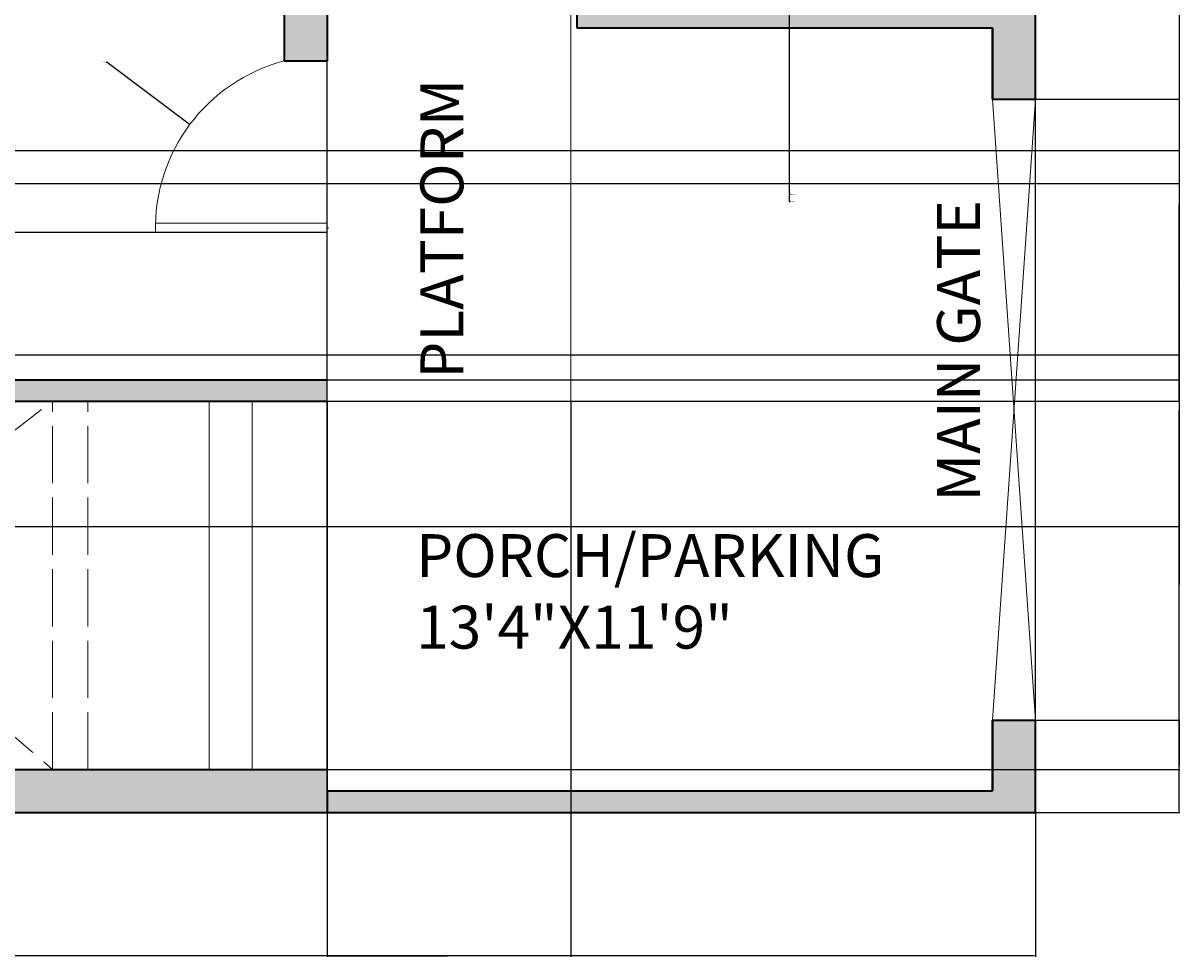
# Model space of a CAD drawing. Units: feet. Extents: x 1699 to 2359, y 1819 to 2211.
# Tile 3 of 4: x 2117 to 2359, y 1819 to 2014. Entities that reach past the tile are written whole.
import ezdxf

# ---------------------------------------------------------------- set-up
doc = ezdxf.new("R2010")
doc.units = ezdxf.units.FT
doc.linetypes.add('ACAD_ISO02W100', pattern=[15, 12, -3])
for name, color, linetype, lineweight in [('A-ANNO-DIMS', 2, 'Continuous', 18), ('A-ANNO-TEXT', 7, 'Continuous', 18), ('A-AREA-IDEN', 7, 'Continuous', 18), ('A-DOOR', 4, 'Continuous', 18), ('A-FLOR', 7, 'Continuous', 18), ('A-FLOR-STRS', 7, 'Continuous', 18), ('A-FLOR-STRS-OVHD', 8, 'ACAD_ISO02W100', 13), ('A-WALL', 7, 'Continuous', 35), ('A-WALL-PATT', 1, 'Continuous', 13)]:
    doc.layers.add(name, color=color, linetype=linetype, lineweight=lineweight)
doc.styles.get("Standard").update_dxf_attribs({"font": 'arial.ttf'})
doc.dimstyles.get("Standard").update_dxf_attribs({"dimtxt": 0.18, "dimasz": 0.18, "dimexe": 0.18, "dimexo": 0.0625, "dimgap": 0.09, "dimtad": 0, "dimtih": 1, "dimtoh": 1, "dimdec": 4, "dimzin": 0, "dimdsep": 46, "dimtxsty": 'Standard', "dimcen": 0.09, "dimadec": 0, "dimazin": 0, "dimtfac": 1, "dimtdec": 4, "dimtofl": 0, "dimtmove": 0, "dimatfit": 3, "dimfxl": 1, "dimtolj": 1, "dimtzin": 0, "dimarcsym": 0})

# ---------------------------------------------------------------- blocks, each defined once
blk = doc.blocks.new('*D22')
at = {"layer": 'A-ANNO-DIMS', "color": 0, "lineweight": -2, "transparency": 16777216}
for p, q in [((2180.43, 1853.41), (2180.43, 2210.63)), ((2180.61, 2210.45), (2254.29, 2210.45)), ((2328.75, 2210.45), (2255.06, 2210.45)), ((2328.93, 1848.91), (2328.93, 2210.63))]:
    blk.add_line(p, q, dxfattribs=at)
at = {"layer": 'A-ANNO-DIMS', "color": 0, "transparency": 16777216}
for points in [[(2180.61, 2210.48), (2180.61, 2210.42), (2180.43, 2210.45)], [(2328.75, 2210.48), (2328.75, 2210.42), (2328.93, 2210.45)]]:
    blk.add_solid(points, dxfattribs=at)
at = {"layer": 'Defpoints', "color": 0, "transparency": 16777216}
for p in [(2328.93, 2210.45), (2180.43, 1853.35), (2328.93, 1848.85)]:
    blk.add_point(p, dxfattribs=at)
at = {"layer": 'A-ANNO-DIMS', "color": 0, "transparency": 16777216, "insert": (2254.68, 2210.45), "char_height": 0.18, "attachment_point": 5}
blk.add_mtext('\\A1;148.5', dxfattribs=at)
blk = doc.blocks.new('*D23')
at = {"layer": 'A-ANNO-DIMS', "color": 0, "lineweight": -2, "transparency": 16777216}
for p, q in [((1955.43, 1857.79), (1955.43, 1818.57)), ((2180.43, 1857.79), (2180.43, 1818.57)), ((1955.61, 1818.75), (2067.64, 1818.75)), ((2180.25, 1818.75), (2068.22, 1818.75))]:
    blk.add_line(p, q, dxfattribs=at)
at = {"layer": 'A-ANNO-DIMS', "color": 0, "transparency": 16777216}
for points in [[(1955.61, 1818.78), (1955.61, 1818.72), (1955.43, 1818.75)], [(2180.25, 1818.78), (2180.25, 1818.72), (2180.43, 1818.75)]]:
    blk.add_solid(points, dxfattribs=at)
at = {"layer": 'Defpoints', "color": 0, "transparency": 16777216}
for p in [(1955.43, 1857.85), (2180.43, 1857.85), (2180.43, 1818.75)]:
    blk.add_point(p, dxfattribs=at)
at = {"layer": 'A-ANNO-DIMS', "color": 0, "transparency": 16777216, "insert": (2067.93, 1818.75), "char_height": 0.18, "attachment_point": 5}
blk.add_mtext('\\A1;225', dxfattribs=at)
blk = doc.blocks.new('*D24')
at = {"layer": 'A-ANNO-DIMS', "color": 0, "lineweight": -2, "transparency": 16777216}
for p, q in [((1955.49, 1935.08), (2359.21, 1935.08)), ((2359.03, 1934.9), (2359.03, 1896.65)), ((2359.03, 1858.03), (2359.03, 1896.28)), ((1955.49, 1857.85), (2359.21, 1857.85))]:
    blk.add_line(p, q, dxfattribs=at)
at = {"layer": 'A-ANNO-DIMS', "color": 0, "transparency": 16777216}
for points in [[(2359, 1934.9), (2359.06, 1934.9), (2359.03, 1935.08)], [(2359, 1858.03), (2359.06, 1858.03), (2359.03, 1857.85)]]:
    blk.add_solid(points, dxfattribs=at)
at = {"layer": 'Defpoints', "color": 0, "transparency": 16777216}
for p in [(1955.43, 1935.08), (2359.03, 1935.08), (1955.43, 1857.85)]:
    blk.add_point(p, dxfattribs=at)
at = {"layer": 'A-ANNO-DIMS', "color": 0, "transparency": 16777216, "insert": (2359.03, 1896.46), "char_height": 0.18, "attachment_point": 5}
blk.add_mtext('\\A1;77.23', dxfattribs=at)
blk = doc.blocks.new('*D28')
at = {"layer": 'A-ANNO-DIMS', "color": 0, "lineweight": -2, "transparency": 16777216}
for p, q in [((2328.99, 1998.37), (2359.21, 1998.37)), ((2359.03, 1998.19), (2359.03, 1933.46)), ((2359.03, 1868.36), (2359.03, 1933.1)), ((2328.99, 1868.18), (2359.21, 1868.18))]:
    blk.add_line(p, q, dxfattribs=at)
at = {"layer": 'A-ANNO-DIMS', "color": 0, "transparency": 16777216}
for points in [[(2359, 1998.19), (2359.06, 1998.19), (2359.03, 1998.37)], [(2359, 1868.36), (2359.06, 1868.36), (2359.03, 1868.18)]]:
    blk.add_solid(points, dxfattribs=at)
at = {"layer": 'Defpoints', "color": 0, "transparency": 16777216}
for p in [(2328.93, 1998.37), (2328.93, 1868.18), (2359.03, 1868.18)]:
    blk.add_point(p, dxfattribs=at)
at = {"layer": 'A-ANNO-DIMS', "color": 0, "transparency": 16777216, "insert": (2359.03, 1933.28), "char_height": 0.18, "attachment_point": 5}
blk.add_mtext('\\A1;130.2', dxfattribs=at)
blk = doc.blocks.new('*D29')
at = {"layer": 'A-ANNO-DIMS', "color": 0, "lineweight": -2, "transparency": 16777216}
for p, q in [((2328.99, 1868.18), (2359.21, 1868.18)), ((2359.03, 1868), (2359.03, 1858.7)), ((2359.03, 1849.03), (2359.03, 1858.33)), ((2328.99, 1848.85), (2359.21, 1848.85))]:
    blk.add_line(p, q, dxfattribs=at)
at = {"layer": 'A-ANNO-DIMS', "color": 0, "transparency": 16777216}
for points in [[(2359, 1868), (2359.06, 1868), (2359.03, 1868.18)], [(2359, 1849.03), (2359.06, 1849.03), (2359.03, 1848.85)]]:
    blk.add_solid(points, dxfattribs=at)
at = {"layer": 'Defpoints', "color": 0, "transparency": 16777216}
for p in [(2328.93, 1868.18), (2328.93, 1848.85), (2359.03, 1848.85)]:
    blk.add_point(p, dxfattribs=at)
at = {"layer": 'A-ANNO-DIMS', "color": 0, "transparency": 16777216, "insert": (2359.03, 1858.52), "char_height": 0.18, "attachment_point": 5}
blk.add_mtext('\\A1;19.334', dxfattribs=at)
blk = doc.blocks.new('*D33')
at = {"layer": 'A-ANNO-DIMS', "color": 0, "lineweight": -2, "transparency": 16777216}
for p, q in [((1991.49, 1980.71), (2359.21, 1980.71)), ((2359.03, 1980.53), (2359.03, 1960.33)), ((2359.03, 1939.76), (2359.03, 1959.97)), ((1955.49, 1939.58), (2359.21, 1939.58))]:
    blk.add_line(p, q, dxfattribs=at)
at = {"layer": 'A-ANNO-DIMS', "color": 0, "transparency": 16777216}
for points in [[(2359, 1980.53), (2359.06, 1980.53), (2359.03, 1980.71)], [(2359, 1939.76), (2359.06, 1939.76), (2359.03, 1939.58)]]:
    blk.add_solid(points, dxfattribs=at)
at = {"layer": 'Defpoints', "color": 0, "transparency": 16777216}
for p in [(1991.43, 1980.71), (1955.43, 1939.58), (2359.03, 1939.58)]:
    blk.add_point(p, dxfattribs=at)
at = {"layer": 'A-ANNO-DIMS', "color": 0, "transparency": 16777216, "insert": (2359.03, 1960.15), "char_height": 0.18, "attachment_point": 5}
blk.add_mtext('\\A1;41.14', dxfattribs=at)
blk = doc.blocks.new('*D34')
at = {"layer": 'A-ANNO-DIMS', "color": 0, "lineweight": -2, "transparency": 16777216}
for p, q in [((2180.43, 1935.02), (2180.43, 1818.57)), ((2231.49, 1935.02), (2231.49, 1818.57)), ((2180.61, 1818.75), (2205.57, 1818.75)), ((2231.31, 1818.75), (2206.35, 1818.75))]:
    blk.add_line(p, q, dxfattribs=at)
at = {"layer": 'A-ANNO-DIMS', "color": 0, "transparency": 16777216}
for points in [[(2180.61, 1818.78), (2180.61, 1818.72), (2180.43, 1818.75)], [(2231.31, 1818.78), (2231.31, 1818.72), (2231.49, 1818.75)]]:
    blk.add_solid(points, dxfattribs=at)
at = {"layer": 'Defpoints', "color": 0, "transparency": 16777216}
for p in [(2180.43, 1935.08), (2231.49, 1935.08), (2231.49, 1818.75)]:
    blk.add_point(p, dxfattribs=at)
at = {"layer": 'A-ANNO-DIMS', "color": 0, "transparency": 16777216, "insert": (2205.96, 1818.75), "char_height": 0.18, "attachment_point": 5}
blk.add_mtext('\\A1;51.06', dxfattribs=at)
blk = doc.blocks.new('*D35')
at = {"layer": 'A-ANNO-DIMS', "color": 0, "lineweight": -2, "transparency": 16777216}
for p, q in [((2231.55, 2017.45), (2359.21, 2017.45)), ((2359.03, 2017.27), (2359.03, 1976.45)), ((2359.03, 1935.26), (2359.03, 1976.08)), ((2231.55, 1935.08), (2359.21, 1935.08))]:
    blk.add_line(p, q, dxfattribs=at)
at = {"layer": 'A-ANNO-DIMS', "color": 0, "transparency": 16777216}
for points in [[(2359, 2017.27), (2359.06, 2017.27), (2359.03, 2017.45)], [(2359, 1935.26), (2359.06, 1935.26), (2359.03, 1935.08)]]:
    blk.add_solid(points, dxfattribs=at)
at = {"layer": 'Defpoints', "color": 0, "transparency": 16777216}
for p in [(2231.49, 2017.45), (2359.03, 2017.45), (2231.49, 1935.08)]:
    blk.add_point(p, dxfattribs=at)
at = {"layer": 'A-ANNO-DIMS', "color": 0, "transparency": 16777216, "insert": (2359.03, 1976.26), "char_height": 0.18, "attachment_point": 5}
blk.add_mtext('\\A1;82.37', dxfattribs=at)
blk = doc.blocks.new('*D38')
at = {"layer": 'A-ANNO-DIMS', "color": 0, "lineweight": -2, "transparency": 16777216}
for p, q in [((1784.49, 1944.78), (2359.21, 1944.78)), ((2359.03, 1944.6), (2359.03, 1926.96)), ((2359.03, 1908.96), (2359.03, 1926.6)), ((1784.49, 1908.78), (2359.21, 1908.78))]:
    blk.add_line(p, q, dxfattribs=at)
at = {"layer": 'A-ANNO-DIMS', "color": 0, "transparency": 16777216}
for points in [[(2359, 1944.6), (2359.06, 1944.6), (2359.03, 1944.78)], [(2359, 1908.96), (2359.06, 1908.96), (2359.03, 1908.78)]]:
    blk.add_solid(points, dxfattribs=at)
at = {"layer": 'Defpoints', "color": 0, "transparency": 16777216}
for p in [(1784.43, 1944.78), (2359.03, 1944.78), (1784.43, 1908.78)]:
    blk.add_point(p, dxfattribs=at)
at = {"layer": 'A-ANNO-DIMS', "color": 0, "transparency": 16777216, "insert": (2359.03, 1926.78), "char_height": 0.18, "attachment_point": 5}
blk.add_mtext('\\A1;36', dxfattribs=at)
blk = doc.blocks.new('*D39')
at = {"layer": 'A-ANNO-DIMS', "color": 0, "lineweight": -2, "transparency": 16777216}
for p, q in [((1784.49, 1987.61), (2359.21, 1987.61)), ((2359.03, 1987.43), (2359.03, 1966.38)), ((2359.03, 1944.96), (2359.03, 1966.02)), ((1784.49, 1944.78), (2359.21, 1944.78))]:
    blk.add_line(p, q, dxfattribs=at)
at = {"layer": 'A-ANNO-DIMS', "color": 0, "transparency": 16777216}
for points in [[(2359, 1987.43), (2359.06, 1987.43), (2359.03, 1987.61)], [(2359, 1944.96), (2359.06, 1944.96), (2359.03, 1944.78)]]:
    blk.add_solid(points, dxfattribs=at)
at = {"layer": 'Defpoints', "color": 0, "transparency": 16777216}
for p in [(1784.43, 1987.61), (2359.03, 1987.61), (1784.43, 1944.78)]:
    blk.add_point(p, dxfattribs=at)
at = {"layer": 'A-ANNO-DIMS', "color": 0, "transparency": 16777216, "insert": (2359.03, 1966.2), "char_height": 0.18, "attachment_point": 5}
blk.add_mtext('\\A1;42.83', dxfattribs=at)
blk = doc.blocks.new('*D40')
at = {"layer": 'A-ANNO-DIMS', "color": 0, "lineweight": -2, "transparency": 16777216}
for p, q in [((1729.43, 1848.79), (1729.43, 1818.57)), ((2328.93, 1848.79), (2328.93, 1818.57)), ((1729.61, 1818.75), (2028.78, 1818.75)), ((2328.75, 1818.75), (2029.57, 1818.75))]:
    blk.add_line(p, q, dxfattribs=at)
at = {"layer": 'A-ANNO-DIMS', "color": 0, "transparency": 16777216}
for points in [[(1729.61, 1818.78), (1729.61, 1818.72), (1729.43, 1818.75)], [(2328.75, 1818.78), (2328.75, 1818.72), (2328.93, 1818.75)]]:
    blk.add_solid(points, dxfattribs=at)
at = {"layer": 'Defpoints', "color": 0, "transparency": 16777216}
for p in [(1729.43, 1848.85), (2328.93, 1848.85), (2328.93, 1818.75)]:
    blk.add_point(p, dxfattribs=at)
at = {"layer": 'A-ANNO-DIMS', "color": 0, "transparency": 16777216, "insert": (2029.18, 1818.75), "char_height": 0.18, "attachment_point": 5}
blk.add_mtext('\\A1;599.5', dxfattribs=at)
blk = doc.blocks.new('*D48')
at = {"layer": 'A-ANNO-DIMS', "color": 0, "lineweight": -2, "transparency": 16777216}
for p, q in [((2180.36, 1970.41), (1699.15, 1970.41)), ((1699.33, 1970.23), (1699.33, 1955.18)), ((1699.33, 1939.76), (1699.33, 1954.81)), ((2180.36, 1939.58), (1699.15, 1939.58))]:
    blk.add_line(p, q, dxfattribs=at)
at = {"layer": 'A-ANNO-DIMS', "color": 0, "transparency": 16777216}
for points in [[(1699.3, 1970.23), (1699.36, 1970.23), (1699.33, 1970.41)], [(1699.3, 1939.76), (1699.36, 1939.76), (1699.33, 1939.58)]]:
    blk.add_solid(points, dxfattribs=at)
at = {"layer": 'Defpoints', "color": 0, "transparency": 16777216}
for p in [(1699.33, 1970.41), (2180.43, 1970.41), (2180.43, 1939.58)]:
    blk.add_point(p, dxfattribs=at)
at = {"layer": 'A-ANNO-DIMS', "color": 0, "transparency": 16777216, "insert": (1699.33, 1954.99), "char_height": 0.18, "attachment_point": 5}
blk.add_mtext('\\A1;30.833', dxfattribs=at)
blk = doc.blocks.new('*D56')
at = {"layer": 'A-ANNO-DIMS', "color": 0, "lineweight": -2, "transparency": 16777216}
for p, q in [((2134.1, 2006.15), (2134.28, 2006.15)), ((2134.28, 2006.15), (2151.51, 1993.23)), ((2180.5, 1971.41), (2180.68, 1971.41)), ((2180.59, 1971.32), (2180.59, 1971.5))]:
    blk.add_line(p, q, dxfattribs=at)
at = {"layer": 'A-ANNO-DIMS', "color": 0, "transparency": 16777216}
blk.add_solid([(2151.52, 1993.25), (2151.49, 1993.2), (2151.65, 1993.12)], dxfattribs=at)
at = {"layer": 'Defpoints', "color": 0, "transparency": 16777216}
for p in [(2151.65, 1993.12), (2180.59, 1971.41)]:
    blk.add_point(p, dxfattribs=at)
at = {"layer": 'A-ANNO-DIMS', "color": 0, "transparency": 16777216, "insert": (2133.62, 2006.15), "char_height": 0.18, "attachment_point": 5}
blk.add_mtext('\\A1;R36.18', dxfattribs=at)
blk = doc.blocks.new('*D59')
at = {"layer": 'A-ANNO-DIMS', "color": 0, "lineweight": -2, "transparency": 16777216}
for p, q in [((2277.29, 2140.01), (2277.47, 2140.01)), ((2277.38, 2139.92), (2277.38, 2140.1)), ((2277.38, 1978.42), (2277.38, 2038.84)), ((2277.56, 1978.42), (2277.38, 1978.42))]:
    blk.add_line(p, q, dxfattribs=at)
at = {"layer": 'A-ANNO-DIMS', "color": 0, "transparency": 16777216}
blk.add_solid([(2277.41, 2038.84), (2277.35, 2038.84), (2277.38, 2039.02)], dxfattribs=at)
at = {"layer": 'Defpoints', "color": 0, "transparency": 16777216}
for p in [(2277.38, 2140.01), (2277.38, 2039.02)]:
    blk.add_point(p, dxfattribs=at)
at = {"layer": 'A-ANNO-DIMS', "color": 0, "transparency": 16777216, "insert": (2278.11, 1978.42), "char_height": 0.18, "attachment_point": 5}
blk.add_mtext('\\A1;2X R101', dxfattribs=at)
blk = doc.blocks.new('*D60')
at = {"layer": 'A-ANNO-DIMS', "color": 0, "lineweight": -2, "transparency": 16777216}
for p, q in [((2277.29, 2129.22), (2277.47, 2129.22)), ((2277.38, 2129.13), (2277.38, 2129.31)), ((2277.38, 1976.89), (2277.38, 2033.84)), ((2277.56, 1976.89), (2277.38, 1976.89))]:
    blk.add_line(p, q, dxfattribs=at)
at = {"layer": 'A-ANNO-DIMS', "color": 0, "transparency": 16777216}
blk.add_solid([(2277.41, 2033.84), (2277.35, 2033.84), (2277.38, 2034.02)], dxfattribs=at)
at = {"layer": 'Defpoints', "color": 0, "transparency": 16777216}
for p in [(2277.38, 2129.22), (2277.38, 2034.02)]:
    blk.add_point(p, dxfattribs=at)
at = {"layer": 'A-ANNO-DIMS', "color": 0, "transparency": 16777216, "insert": (2278.16, 1976.89), "char_height": 0.18, "attachment_point": 5}
blk.add_mtext('\\A1;2X R95.2', dxfattribs=at)

msp = doc.modelspace()

# ---------------------------------------------------------------- hatches: boundary and pattern name
at = {"layer": 'A-WALL-PATT'}
h = msp.add_hatch(color=256, dxfattribs=at)
h.dxf.hatch_style = 1
h.paths.add_polyline_path([(2180.4267, 1853.3494), (2180.4267, 1857.8494), (1955.4267, 1857.8494), (1955.4267, 1935.0782), (1991.4267, 1935.0782), (1991.4267, 1939.5782), (1955.4267, 1939.5782), (1955.4267, 2022.8494), (1950.9267, 2022.8494), (1950.9267, 1857.8494), (1784.4267, 1857.8494), (1784.4267, 1908.7829), (1775.4267, 1908.7829), (1775.4267, 1853.3494), (1733.9267, 1853.3494), (1733.9267, 2018.3494), (1775.4267, 2018.3494), (1775.4267, 2022.8494), (1738.4267, 2022.8494), (1738.4267, 2171.3494), (1898.4267, 2171.3494), (1898.4267, 2060.8494), (1902.9267, 2060.8494), (1902.9267, 2064.8494), (1955.4267, 2064.8494), (1955.4267, 2069.3494), (1902.9267, 2069.3494), (1902.9267, 2171.3494), (1950.9267, 2171.3494), (1950.9267, 2169.0373), (1955.4267, 2169.0373), (1955.4267, 2175.8494), (2114.4267, 2175.8494), (2114.4267, 2167.1408), (2118.9267, 2167.1408), (2118.9267, 2171.3494), (2166.9267, 2171.3494), (2166.9267, 2113.3494), (2171.4267, 2113.3494), (2171.4267, 2171.3494), (2319.9267, 2171.3494), (2319.9267, 2132.5785), (2328.9267, 2132.5785), (2328.9267, 2180.3494), (2309.4267, 2180.3494), (1729.4267, 2180.3494), (1729.4267, 1848.8494), (2180.4267, 1848.8494)])
h.paths.add_polyline_path([(1784.4267, 1987.6139), (1775.4267, 1987.6139), (1775.4267, 1944.7829), (1784.4267, 1944.7829)], flags=17)
h.paths.add_polyline_path([(1912.9267, 2022.8494), (1775.4267, 2022.8494), (1775.4267, 2013.6139), (1784.4267, 2013.6139), (1784.4267, 2018.3494), (1912.9267, 2018.3494)], flags=17)
h.paths.add_polyline_path([(2018.4267, 2135.3494), (2047.4307, 2135.3494), (2047.4307, 2139.8494), (1981.4267, 2139.8494), (1981.4267, 2135.3494), (2013.9267, 2135.3494), (2013.9267, 2059.8494), (2018.4267, 2059.8494)], flags=17)
h.paths.add_polyline_path([(2114.4267, 2139.8494), (2071.4307, 2139.8494), (2071.4307, 2135.3494), (2114.4267, 2135.3494)], flags=17)
h.paths.add_polyline_path([(2118.9267, 2143.1408), (2114.4267, 2143.1408), (2114.4267, 2059.8494), (2118.9267, 2059.8494), (2118.9267, 2082.8494), (2184.631, 2082.8494), (2184.631, 2087.3494), (2118.9267, 2087.3494)], flags=17)
h.paths.add_polyline_path([(2328.9267, 2084.5785), (2319.9267, 2084.5785), (2319.9267, 2022.8494), (2232.7955, 2022.8494), (2232.7955, 2013.3494), (2319.9267, 2013.3494), (2319.9267, 1998.3723), (2328.9267, 1998.3723)], flags=17)
h.paths.add_polyline_path([(2180.4267, 2043.5261), (2171.4267, 2043.5261), (2171.4267, 2006.4114), (2180.4267, 2006.4114)], flags=17)
h.paths.add_polyline_path([(2015.0526, 1939.5782), (1991.4267, 1939.5782), (1991.4267, 1935.0782), (2015.0526, 1935.0782)], flags=17)
h.paths.add_polyline_path([(2180.4267, 1939.5782), (2087.0526, 1939.5782), (2087.0526, 1935.0782), (2180.4267, 1935.0782)], flags=17)
h.paths.add_polyline_path([(2328.9267, 1868.1839), (2319.9267, 1868.1839), (2319.9267, 1853.3494), (2180.4267, 1853.3494), (2180.4267, 1848.8494), (2328.9267, 1848.8494)], flags=17)

# ---------------------------------------------------------------- linework, layer by layer
at = {"layer": 'A-DOOR'}
for p, q in [((2319.9267, 1868.1839), (2328.9267, 1998.3723)), ((2328.9267, 1868.1839), (2319.9267, 1998.3723)), ((2144.4267, 1970.4114), (2144.4267, 1972.4114)), ((2144.4267, 1972.4114), (2180.4267, 1972.4114)), ((2180.4267, 1970.4114), (2144.4267, 1970.4114)), ((2180.4267, 1970.4114), (2144.4267, 1970.4114))]:
    msp.add_line(p, q, dxfattribs=at)
msp.add_arc((2180.5933, 1971.4114), 36.1805, 104.676393, 181.583812, dxfattribs=at)
at = {"layer": 'A-FLOR'}
for p, q in [((2231.4915, 1935.0782), (2231.4915, 2017.4514)), ((2180.4267, 2006.4114), (2180.4267, 1853.3494)), ((2180.4267, 1935.0782), (2231.4915, 1935.0782))]:
    msp.add_line(p, q, dxfattribs=at)
at = {"layer": 'A-FLOR-STRS'}
for p, q in [((2155.6612, 1857.8494), (2155.6612, 1935.0782)), ((2164.6763, 1857.8494), (2164.6763, 1935.0782))]:
    msp.add_line(p, q, dxfattribs=at)
at = {"layer": 'A-FLOR-STRS-OVHD'}
for p, q in [((2075.4267, 1898.4702), (2122.862, 1935.0782)), ((2122.862, 1857.8494), (2122.862, 1935.0782)), ((2130.2688, 1857.8494), (2130.2688, 1935.0782)), ((2075.4267, 1898.4702), (2122.862, 1857.8494))]:
    msp.add_line(p, q, dxfattribs=at)
at = {"layer": 'A-WALL'}
for p, q in [((2328.9267, 1998.3723), (2328.9267, 2180.2967)), ((2171.4267, 2043.5261), (2171.4267, 2006.4114)), ((2180.4267, 2043.5261), (2180.4267, 2006.4114)), ((2232.7955, 2022.8494), (2232.7955, 2013.3494)), ((2232.7955, 2013.3494), (2319.9267, 2013.3494)), ((2319.9267, 2013.3494), (2319.9267, 1998.3723)), ((2319.9267, 1998.3723), (2319.9267, 2013.3494)), ((2171.4267, 2006.4114), (2180.4267, 2006.4114)), ((2319.9267, 1998.3723), (2328.9267, 1998.3723)), ((1955.4267, 1939.5782), (2180.4267, 1939.5782)), ((1955.4267, 1935.0782), (2180.4267, 1935.0782)), ((2319.9267, 1853.3494), (2319.9267, 1868.1839)), ((2319.9267, 1868.1839), (2328.9267, 1868.1839)), ((2319.9267, 1868.1839), (2319.9267, 1853.3494)), ((2328.9267, 1848.8494), (2328.9267, 1868.1839)), ((1955.4267, 1857.8494), (2180.4267, 1857.8494)), ((2180.4267, 1853.3494), (2180.4267, 1848.8494)), ((2180.4267, 1853.3494), (2319.9267, 1853.3494)), ((1729.4267, 1848.8494), (2328.9267, 1848.8494))]:
    msp.add_line(p, q, dxfattribs=at)

# ---------------------------------------------------------------- texts
at = {"layer": 'A-ANNO-TEXT', "insert": (2308.3041, 1914.0448), "char_height": 9, "attachment_point": 1, "rotation": 90}
msp.add_mtext_dynamic_manual_height_columns('{\\fCambria|b0|i0|c0|p18;MAIN GATE}', width=105.143232, gutter_width=12.5, heights=[0], dxfattribs=at)
at = {"layer": 'A-AREA-IDEN', "insert": (2199.9708, 1939.7846), "char_height": 9, "attachment_point": 1, "rotation": 90}
msp.add_mtext_dynamic_manual_height_columns('{\\fCambria|b0|i0|c0|p18;PLATFORM}', width=86.502988, gutter_width=12.5, heights=[29.7261], dxfattribs=at)
at = {"layer": 'A-AREA-IDEN', "insert": (2199.0851, 1907.1905), "char_height": 9, "attachment_point": 1}
msp.add_mtext_dynamic_manual_height_columns('{\\fCambria|b0|i0|c0|p18;PORCH/PARKING\\P13\'4"X11\'9"}', width=66.522428, gutter_width=12.5, heights=[50.97], dxfattribs=at)

# ---------------------------------------------------------------- dimensions: what is measured, and where the dimension line sits
at = {"layer": 'A-ANNO-DIMS'}
for base, p1, p2, override, picture, middle in [((2328.9267, 2210.4494), (2180.4267, 1853.3494), (2328.9267, 1848.8494), {"dimdec": 1, "dimlfac": 1, "dimrnd": 0, "dimzin": 0, "dimdsep": 46, "dimlunit": 2}, '*D22', (2254.6767, 2210.4494)), ((2231.4915, 1818.7494), (2180.4267, 1935.0782), (2231.4915, 1935.0782), {"dimdec": 2, "dimlfac": 1, "dimrnd": 0, "dimzin": 0, "dimdsep": 46, "dimlunit": 2}, '*D34', (2205.9591, 1818.7494)), ((2180.4267, 1818.7494), (1955.4267, 1857.8494), (2180.4267, 1857.8494), {"dimdec": 0, "dimlfac": 1, "dimrnd": 0, "dimzin": 0, "dimdsep": 46, "dimlunit": 2}, '*D23', (2067.9267, 1818.7494)), ((2328.9267, 1818.7494), (1729.4267, 1848.8494), (2328.9267, 1848.8494), {"dimdec": 1, "dimlfac": 1, "dimrnd": 0, "dimzin": 0, "dimdsep": 46, "dimlunit": 2}, '*D40', (2029.1767, 1818.7494))]:
    dim = msp.add_linear_dim(base=base, p1=p1, p2=p2, dimstyle='Standard', override=override, dxfattribs=at)
    dim.commit()
    dim.dimension.update_dxf_attribs({"geometry": picture, "text_midpoint": middle})
for center, mpoint, override, picture, middle in [((2277.3765, 2140.0137), (2277.377, 2039.0163), {"dimdec": 0, "dimlfac": 1, "dimrnd": 0, "dimzin": 0, "dimdsep": 46, "dimlunit": 2}, '*D59', (2278.1098, 1978.4179)), ((2277.3765, 2129.2247), (2277.377, 2034.0163), {"dimdec": 1, "dimlfac": 1, "dimrnd": 0, "dimzin": 0, "dimdsep": 46, "dimlunit": 2}, '*D60', (2278.1612, 1976.8913))]:
    dim = msp.add_radius_dim(center=center, mpoint=mpoint, text='2X <>', dimstyle='Standard', override=override, dxfattribs=at)
    dim.commit()
    dim.dimension.update_dxf_attribs({"geometry": picture, "text_midpoint": middle, "dimtype": 164})
for base, p1, p2, override, picture, middle in [((2359.0267, 2017.4514), (2231.4915, 1935.0782), (2231.4915, 2017.4514), {"dimdec": 2, "dimlfac": 1, "dimrnd": 0, "dimzin": 0, "dimdsep": 46, "dimlunit": 2}, '*D35', (2359.0267, 1976.2648)), ((2359.0267, 1868.1839), (2328.9267, 1998.3723), (2328.9267, 1868.1839), {"dimdec": 1, "dimlfac": 1, "dimrnd": 0, "dimzin": 0, "dimdsep": 46, "dimlunit": 2}, '*D28', (2359.0267, 1933.2781)), ((2359.0267, 1987.6139), (1784.4267, 1944.7829), (1784.4267, 1987.6139), {"dimdec": 2, "dimlfac": 1, "dimrnd": 0, "dimzin": 0, "dimdsep": 46, "dimlunit": 2}, '*D39', (2359.0267, 1966.1984)), ((2359.0267, 1939.5782), (1991.4267, 1980.7142), (1955.4267, 1939.5782), {"dimdec": 2, "dimlfac": 1, "dimrnd": 0, "dimzin": 0, "dimdsep": 46, "dimlunit": 2}, '*D33', (2359.0267, 1960.1462)), ((1699.3267, 1970.4114), (2180.4267, 1939.5782), (2180.4267, 1970.4114), {"dimdec": 3, "dimlfac": 1, "dimrnd": 0, "dimzin": 0, "dimdsep": 46, "dimlunit": 2}, '*D48', (1699.3267, 1954.9948)), ((2359.0267, 1944.7829), (1784.4267, 1908.7829), (1784.4267, 1944.7829), {"dimdec": 0, "dimlfac": 1, "dimrnd": 0, "dimzin": 0, "dimdsep": 46, "dimlunit": 2}, '*D38', (2359.0267, 1926.7829)), ((2359.0267, 1935.0782), (1955.4267, 1857.8494), (1955.4267, 1935.0782), {"dimdec": 2, "dimlfac": 1, "dimrnd": 0, "dimzin": 0, "dimdsep": 46, "dimlunit": 2}, '*D24', (2359.0267, 1896.4638)), ((2359.02665, 1848.84939), (2328.92665, 1868.18386), (2328.92665, 1848.84939), {"dimdec": 3, "dimlfac": 1, "dimrnd": 0, "dimzin": 0, "dimdsep": 46, "dimlunit": 2}, '*D29', (2359.02665, 1858.51662))]:
    dim = msp.add_linear_dim(base=base, p1=p1, p2=p2, angle=90, dimstyle='Standard', override=override, dxfattribs=at)
    dim.commit()
    dim.dimension.update_dxf_attribs({"geometry": picture, "text_midpoint": middle})
dim = msp.add_radius_dim(center=(2180.5933, 1971.4114), mpoint=(2151.6491, 1993.1199), dimstyle='Standard', override={"dimdec": 2, "dimlfac": 1, "dimrnd": 0, "dimzin": 0, "dimdsep": 46, "dimlunit": 2}, dxfattribs=at)
dim.commit()
dim.dimension.update_dxf_attribs({"geometry": '*D56', "text_midpoint": (2133.6225, 2006.145), "dimtype": 164})

doc.saveas('drawing.dxf')
